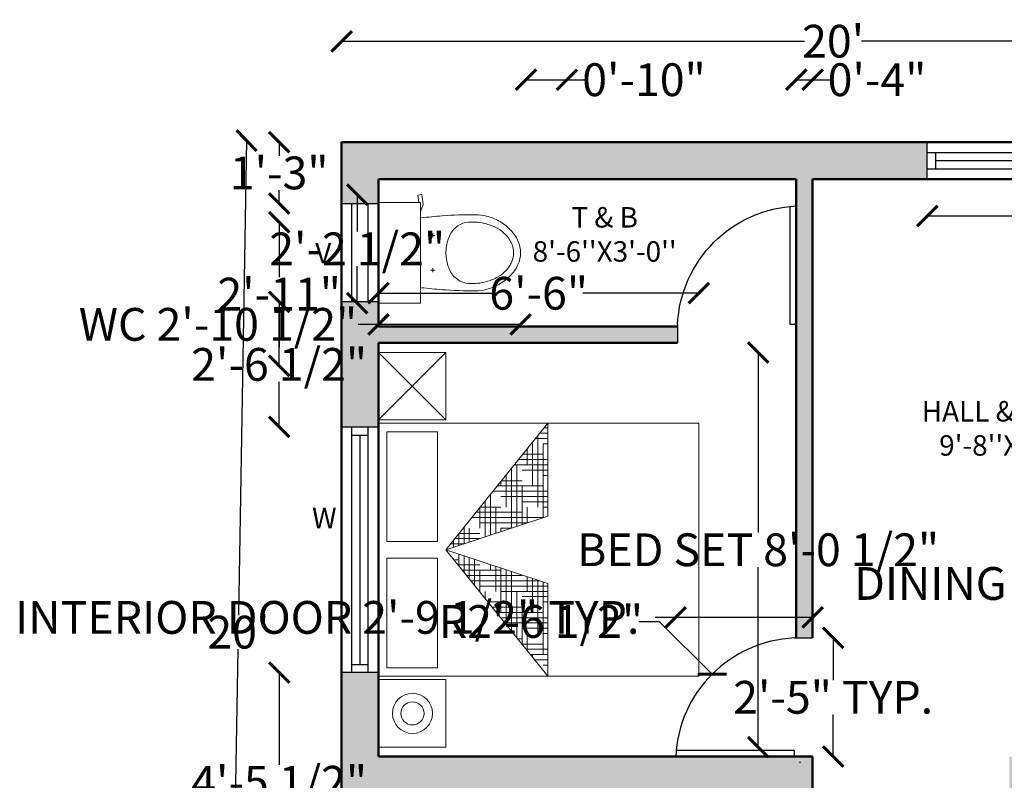
# Model space of a CAD drawing. Units: inches. Extents: x 2015 to 2400, y 1855 to 2156.
# Tile 2 of 3: x 2015 to 2255, y 1971 to 2156. Entities that reach past the tile are written whole.
import ezdxf

# ---------------------------------------------------------------- set-up
doc = ezdxf.new("R2010")
doc.units = ezdxf.units.IN
for name, color, linetype, lineweight in [('A-ANNO-DIMS', 2, 'Continuous', 18), ('A-ANNO-TEXT', 7, 'Continuous', 25), ('A-AREA-IDEN', 7, 'Continuous', 25), ('A-FLOR-FIXT', 9, 'Continuous', 18), ('A-FURN', 8, 'Continuous', 18), ('A-WALL-PATT', 30, 'Continuous', 13), ('Door', 40, 'Continuous', 25), ('Walls', 7, 'Continuous', 50), ('Windows', 150, 'Continuous', 25)]:
    doc.layers.add(name, color=color, linetype=linetype, lineweight=lineweight)
doc.styles.get("Standard").update_dxf_attribs({"font": 'arial.ttf'})
doc.dimstyles.get("Standard").update_dxf_attribs({"dimtxt": 8, "dimasz": 5, "dimexe": 0.18, "dimexo": 0.0625, "dimgap": 0.09, "dimtad": 0, "dimtih": 1, "dimtoh": 1, "dimdec": 1, "dimzin": 0, "dimdsep": 46, "dimlunit": 4, "dimtxsty": 'Standard', "dimblk": 'ARCHTICK', "dimcen": 0.09, "dimse1": 1, "dimse2": 1, "dimadec": 0, "dimazin": 0, "dimtfac": 1, "dimtdec": 1, "dimtofl": 0, "dimtmove": 0, "dimatfit": 3, "dimfxl": 1, "dimtolj": 1, "dimtzin": 0, "dimarcsym": 0})

# ---------------------------------------------------------------- blocks, each defined once
blk = doc.blocks.new('*X4')
at = {"color": 0}
for p, q in [((20.199, 14.7812), (20.2772, 14.7812)), ((20.25, 14.8125), (20.2772, 14.8125)), ((20.1487, 14.7188), (20.2772, 14.7188)), ((20.1562, 14.625), (20.1562, 14.7281)), ((20.1739, 14.75), (20.2772, 14.75)), ((20.1875, 14.75), (20.1875, 14.7669)), ((20.25, 14.3194), (20.25, 14.75)), ((20.1236, 14.6875), (20.25, 14.6875)), ((20.125, 14.5), (20.125, 14.6893)), ((20.0625, 14.2573), (20.0625, 14.6116)), ((20.0938, 14.375), (20.0938, 14.6504)), ((20.0984, 14.6562), (20.125, 14.6562)), ((20.2188, 14.3091), (20.2188, 14.625)), ((20.25, 14.625), (20.2772, 14.625)), ((20.023, 14.5625), (20.2772, 14.5625)), ((20.0312, 14.2469), (20.0312, 14.5727)), ((20.125, 14.5938), (20.2772, 14.5938)), ((19.9727, 14.5), (20.25, 14.5)), ((19.9979, 14.5312), (20.2772, 14.5312)), ((20, 14.2366), (20, 14.5)), ((20.1875, 14.2987), (20.1875, 14.5)), ((19.9225, 14.4375), (20, 14.4375)), ((19.9476, 14.4688), (20.125, 14.4688)), ((20.25, 14.4375), (20.2772, 14.4375)), ((19.875, 14.25), (19.875, 14.3785)), ((19.9062, 14.375), (19.9062, 14.4174)), ((19.9688, 14.2262), (19.9688, 14.375)), ((20, 14.375), (20.2772, 14.375)), ((20.125, 14.4062), (20.2772, 14.4062)), ((20.1562, 14.2884), (20.1562, 14.375)), ((19.8219, 14.3125), (20.2291, 14.3125)), ((19.8438, 14.1848), (19.8438, 14.3397)), ((19.875, 14.3438), (20.2772, 14.3438)), ((19.7716, 14.25), (20, 14.25)), ((19.7812, 14.1641), (19.7812, 14.262)), ((19.7967, 14.2812), (20.125, 14.2812)), ((19.8125, 14.1744), (19.8125, 14.3008)), ((19.9375, 14.2159), (19.9375, 14.25)), ((19.7465, 14.2188), (19.875, 14.2188)), ((19.75, 14.1537), (19.75, 14.2231)), ((19.7213, 14.1875), (19.75, 14.1875)), ((19.7018, 14.0938), (19.7786, 14.0938)), ((19.7188, 14.0726), (19.7188, 14.1136)), ((19.75, 14.0338), (19.75, 14.1032)), ((19.7812, 13.9949), (19.7812, 14.0929)), ((19.8125, 14), (19.8125, 14.0825)), ((19.7269, 14.0625), (19.8728, 14.0625)), ((19.752, 14.0312), (19.875, 14.0312)), ((19.9062, 13.8396), (19.9062, 14.0514)), ((19.9375, 13.8007), (19.9375, 14.0411)), ((19.9688, 13.875), (19.9688, 14.0307)), ((20, 14), (20, 14.0204)), ((19.875, 13.8784), (19.875, 14)), ((19.875, 13.9688), (20.1557, 13.9688)), ((20, 14), (20.0614, 14)), ((20.0625, 13.6454), (20.0625, 13.9996)), ((20.0938, 13.625), (20.0938, 13.9893)), ((20.125, 13.75), (20.125, 13.9789)), ((20.1562, 13.875), (20.1562, 13.9686)), ((19.8275, 13.9375), (20.25, 13.9375)), ((19.8526, 13.9062), (20.125, 13.9062)), ((20.25, 13.5), (20.25, 13.9375)), ((19.8777, 13.875), (20, 13.875)), ((20.0312, 13.6842), (20.0312, 13.875)), ((20.125, 13.8438), (20.2772, 13.8438)), ((20.2188, 13.4511), (20.2188, 13.875)), ((20.25, 13.875), (20.2772, 13.875)), ((19.9532, 13.7812), (20.2772, 13.7812)), ((20, 13.8125), (20.2772, 13.8125)), ((19.9783, 13.75), (20.25, 13.75)), ((20, 13.723), (20, 13.75)), ((20.1875, 13.49), (20.1875, 13.75)), ((20.0035, 13.7188), (20.125, 13.7188)), ((20.25, 13.6875), (20.2772, 13.6875)), ((20.0789, 13.625), (20.2772, 13.625)), ((20.125, 13.6562), (20.2772, 13.6562)), ((20.1562, 13.5288), (20.1562, 13.625)), ((20.104, 13.5938), (20.2772, 13.5938)), ((20.1292, 13.5625), (20.25, 13.5625)), ((20.25, 13.5), (20.2772, 13.5)), ((20.2046, 13.4688), (20.2772, 13.4688)), ((20.2297, 13.4375), (20.2772, 13.4375)), ((20.2549, 13.4062), (20.2772, 13.4062))]:
    blk.add_line(p, q, dxfattribs=at)
blk = doc.blocks.new('MAT-P13')
for p, q in [((-1.17, 0), (-1.17, -0.4)), ((-1.17, 0), (-0.77, 0)), ((-0.77, 0), (-0.77, -0.4)), ((-0.75, 0), (0.75, 0)), ((-0.75, 0), (-0.75, -1.9)), ((0.75, 0), (0.75, -1.9)), ((0.77, 0), (1.17, 0)), ((0.77, 0), (0.77, -0.4)), ((0.77, -0.4), (1.17, 0)), ((1.17, -0.4), (0.77, 0)), ((1.17, 0), (1.17, -0.4)), ((-0.7, -0.05), (-0.7, -0.35)), ((-0.7, -0.05), (-0.05, -0.05)), ((-0.05, -0.35), (-0.05, -0.05)), ((0.05, -0.05), (0.7, -0.05)), ((0.05, -0.35), (0.05, -0.05)), ((0.7, -0.05), (0.7, -0.35)), ((-0.7, -0.35), (-0.05, -0.35)), ((0.05, -0.35), (0.7, -0.35)), ((-1.17, -0.4), (-0.77, -0.4)), ((-0.75, -1.0034), (0, -0.4)), ((0, -0.4), (-0.75, -1.0034)), ((0, -0.4), (-0.2, -1.0034)), ((0, -0.4), (0.2, -1.0034)), ((0, -0.4), (0.75, -1.0034)), ((0.77, -0.4), (1.17, -0.4)), ((-0.75, -1.0034), (-0.2, -1.0034)), ((0.2, -1.0034), (0.75, -1.0034)), ((0.75, -1.9), (-0.75, -1.9))]:
    blk.add_line(p, q)
for radius in [0.1189, 0.0686]:
    blk.add_circle((-0.97, -0.2016), radius)
at = {"xscale": -1, "rotation": 90}
blk.add_blockref('*X4', (14.1285, 19.2738), dxfattribs=at)
blk = doc.blocks.new('AP0B05')
for p, q in [((35, 100), (35, 880)), ((75, 100), (75, 878.9)), ((35, 100), (35, -20)), ((815, 100), (815, -20))]:
    blk.add_line(p, q)
blk.add_lwpolyline([(35, 100), (75, 100)])
blk.add_arc((-2.4, 62.6), 818.3, 2.62122, 87.37878)
blk = doc.blocks.new('toilet-1')
at = {"color": 0, "linetype": 'ByBlock'}
for p, q in [((-0.23, -0.02), (-0.23, -0.2116)), ((0.23, -0.02), (-0.23, -0.02)), ((0.23, -0.02), (0.23, -0.2116)), ((-0.23, -0.2116), (0.23, -0.2116)), ((0.1917, -0.2144), (0.2206, -0.225)), ((0.2206, -0.225), (0.266, -0.2187)), ((0.2633, -0.1997), (0.23, -0.2044)), ((0.266, -0.2187), (0.2633, -0.1997)), ((-0.0889, -0.2683), (-0.0697, -0.2683)), ((-0.0793, -0.2587), (-0.0793, -0.2778)), ((0.0889, -0.2683), (0.0698, -0.2683)), ((0.0794, -0.2587), (0.0794, -0.2778)), ((0, -0.6382), (0, -0.6382))]:
    blk.add_line(p, q, dxfattribs=at)
for centre, radius, start, end in [((3.5272, -0.6239), 3.7093, 173.6925, 175.1593), ((-3.527, -0.624), 3.7093, 4.8413, 6.3171), ((1.7368, -0.4519), 1.9109, 175.7698, 180.3758), ((-1.7366, -0.4519), 1.9109, 359.6242, 4.2302), ((-0.0312, -0.4465), 0.1114, 113.8997, 145.1485), ((0, -0.5169), 0.1884, 66.0939, 113.9061), ((0.0312, -0.4465), 0.1114, 34.8515, 66.1003), ((-0.0408, -0.4398), 0.0996, 145.1497, 175.881), ((0.0409, -0.4398), 0.0996, 4.119, 34.8503), ((0.0981, -0.4497), 0.2389, 175.8862, 195.5931), ((-0.098, -0.4497), 0.2389, 344.4069, 4.1138), ((0.0353, -0.463), 0.2093, 180.3747, 194.3375), ((-0.0351, -0.463), 0.2093, 345.6614, 359.6243), ((0.055, -0.458), 0.2297, 194.3353, 209.622), ((0.0961, -0.4503), 0.2369, 195.5969, 209.3771), ((-0.096, -0.4503), 0.2369, 330.6229, 344.4031), ((-0.0548, -0.458), 0.2297, 330.3788, 345.6655), ((0.0647, -0.4524), 0.2409, 209.6273, 224.5489), ((0.0232, -0.4913), 0.1532, 209.3871, 226.5438), ((-0.0231, -0.4913), 0.1532, 313.4562, 330.6129), ((-0.0645, -0.4524), 0.2409, 315.4504, 330.372), ((0.0178, -0.4986), 0.1751, 224.552, 245.714), ((0.0152, -0.4997), 0.1416, 226.5501, 246.5527), ((0, -0.5347), 0.1034, 246.5493, 270.0042), ((0, -0.5347), 0.1034, 269.9958, 293.4507), ((-0.0151, -0.4997), 0.1416, 293.4473, 313.4499), ((-0.0176, -0.4986), 0.1751, 294.2865, 315.4485), ((0.0004, -0.538), 0.132, 245.5845, 269.8782), ((-0.0002, -0.538), 0.132, 270.1216, 294.4153)]:
    blk.add_arc(centre, radius, start, end, dxfattribs=at)
blk = doc.blocks.new('_ArchTick')
at = {"color": 0, "linetype": 'ByBlock', "const_width": 0.15}
blk.add_lwpolyline([(-0.5, -0.5), (0.5, 0.5)], dxfattribs=at)
blk = doc.blocks.new('*D12')
at = {"layer": 'A-ANNO-DIMS', "color": 0, "lineweight": -2, "transparency": 16777216}
for p, q in [((2093.14, 2151.23), (2206.19, 2151.23)), ((2333.14, 2151.23), (2220.09, 2151.23))]:
    blk.add_line(p, q, dxfattribs=at)
at = {"layer": 'Defpoints', "color": 0, "transparency": 16777216}
for p in [(2333.14, 2151.23), (2093.14, 2126.58), (2333.14, 2126.58)]:
    blk.add_point(p, dxfattribs=at)
at = {"layer": 'A-ANNO-DIMS', "color": 0, "lineweight": -2, "transparency": 16777216, "xscale": 5, "yscale": 5, "zscale": 5, "rotation": 180}
blk.add_blockref('_ArchTick', (2093.14, 2151.23), dxfattribs=at)
at = {"layer": 'A-ANNO-DIMS', "color": 0, "lineweight": -2, "transparency": 16777216, "xscale": 5, "yscale": 5, "zscale": 5}
blk.add_blockref('_ArchTick', (2333.14, 2151.23), dxfattribs=at)
at = {"layer": 'A-ANNO-DIMS', "color": 0, "transparency": 16777216, "insert": (2213.14, 2151.23), "char_height": 8, "attachment_point": 5}
blk.add_mtext("\\A1;20'", dxfattribs=at)
blk = doc.blocks.new('*D13')
at = {"layer": 'A-ANNO-DIMS', "color": 0, "lineweight": -2, "transparency": 16777216}
for p, q in [((2069.93, 2126.97), (2067.99, 2011.14)), ((2065.91, 1886.97), (2067.85, 2002.79))]:
    blk.add_line(p, q, dxfattribs=at)
at = {"layer": 'Defpoints', "color": 0, "transparency": 16777216}
for p in [(2093.14, 2126.58), (2065.91, 1886.97), (2089.12, 1886.58)]:
    blk.add_point(p, dxfattribs=at)
at = {"layer": 'A-ANNO-DIMS', "color": 0, "lineweight": -2, "transparency": 16777216, "xscale": 5, "yscale": 5, "zscale": 5}
for p, rotation in [((2069.93, 2126.97), 89.03988190259393), ((2065.91, 1886.97), 269.039881902594)]:
    blk.add_blockref('_ArchTick', p, dxfattribs=dict(at, rotation=rotation))
at = {"layer": 'A-ANNO-DIMS', "color": 0, "transparency": 16777216, "insert": (2067.92, 2006.97), "char_height": 8, "attachment_point": 5}
blk.add_mtext("\\A1;20'", dxfattribs=at)
blk = doc.blocks.new('WIN-60IN')
for p, q in [((0, 6.5), (60, 6.5)), ((2, 6.5), (2, 2.5)), ((58, 6.5), (58, 2.5)), ((0, 2.5), (60, 2.5)), ((2, 4.5), (58, 4.5))]:
    blk.add_line(p, q)
blk.add_lwpolyline([(0, 9), (60, 9), (60, 0), (0, 0)], close=True)
blk = doc.blocks.new('WIN-24IN')
for p, q in [((2.5, 0), (2.5, 24)), ((6.5, 0), (6.5, 24))]:
    blk.add_line(p, q)
blk.add_lwpolyline([(0, 0), (0, 24), (9, 24), (9, 0)], close=True)
blk = doc.blocks.new('*D17')
at = {"layer": 'A-ANNO-DIMS', "color": 0, "lineweight": -2, "transparency": 16777216}
for p, q in [((2174.71, 2010.57), (2169.71, 2010.57)), ((2208.14, 2010.57), (2174.71, 2010.57))]:
    blk.add_line(p, q, dxfattribs=at)
at = {"layer": 'Defpoints', "color": 0, "transparency": 16777216}
for p in [(2174.71, 2010.57), (2174.71, 2005.56), (2208.14, 2005.56)]:
    blk.add_point(p, dxfattribs=at)
at = {"layer": 'A-ANNO-DIMS', "color": 0, "lineweight": -2, "transparency": 16777216, "xscale": 5, "yscale": 5, "zscale": 5, "rotation": 180}
blk.add_blockref('_ArchTick', (2174.71, 2010.57), dxfattribs=at)
at = {"layer": 'A-ANNO-DIMS', "color": 0, "lineweight": -2, "transparency": 16777216, "xscale": 5, "yscale": 5, "zscale": 5}
blk.add_blockref('_ArchTick', (2208.14, 2010.57), dxfattribs=at)
at = {"layer": 'A-ANNO-DIMS', "color": 0, "transparency": 16777216, "insert": (2089.64, 2010.57), "char_height": 8, "attachment_point": 5}
blk.add_mtext('\\A1;INTERIOR DOOR 2\'-9 1/2" TYP.', dxfattribs=at)
blk = doc.blocks.new('*D18')
at = {"layer": 'A-ANNO-DIMS', "color": 0, "lineweight": -2, "transparency": 16777216}
for p, q in [((2213.15, 2005.56), (2213.15, 1995.24)), ((2213.15, 1976.58), (2213.15, 1986.89))]:
    blk.add_line(p, q, dxfattribs=at)
at = {"layer": 'Defpoints', "color": 0, "transparency": 16777216}
for p in [(2208.14, 2005.56), (2213.15, 2005.56), (2208.14, 1976.58)]:
    blk.add_point(p, dxfattribs=at)
at = {"layer": 'A-ANNO-DIMS', "color": 0, "lineweight": -2, "transparency": 16777216, "xscale": 5, "yscale": 5, "zscale": 5}
for p, rotation in [((2213.15, 2005.56), 90), ((2213.15, 1976.58), 270)]:
    blk.add_blockref('_ArchTick', p, dxfattribs=dict(at, rotation=rotation))
at = {"layer": 'A-ANNO-DIMS', "color": 0, "transparency": 16777216, "insert": (2213.15, 1991.07), "char_height": 8, "attachment_point": 5}
blk.add_mtext('\\A1;2\'-5" TYP.', dxfattribs=at)
blk = doc.blocks.new('*D19')
at = {"layer": 'A-ANNO-DIMS', "color": 0, "lineweight": -2, "transparency": 16777216}
for p, q in [((2236.14, 2108.58), (2296.14, 2108.58)), ((2296.14, 2108.58), (2301.14, 2108.58))]:
    blk.add_line(p, q, dxfattribs=at)
at = {"layer": 'Defpoints', "color": 0, "transparency": 16777216}
for p in [(2236.14, 2117.58), (2296.14, 2117.58), (2296.14, 2108.58)]:
    blk.add_point(p, dxfattribs=at)
at = {"layer": 'A-ANNO-DIMS', "color": 0, "lineweight": -2, "transparency": 16777216, "xscale": 5, "yscale": 5, "zscale": 5, "rotation": 180}
blk.add_blockref('_ArchTick', (2236.14, 2108.58), dxfattribs=at)
at = {"layer": 'A-ANNO-DIMS', "color": 0, "lineweight": -2, "transparency": 16777216, "xscale": 5, "yscale": 5, "zscale": 5}
blk.add_blockref('_ArchTick', (2296.14, 2108.58), dxfattribs=at)
at = {"layer": 'A-ANNO-DIMS', "color": 0, "transparency": 16777216, "insert": (2351.85, 2108.58), "char_height": 8, "attachment_point": 5}
blk.add_mtext('\\A1;WINDOW 5\'-0" TYP.', dxfattribs=at)
blk = doc.blocks.new('*D27')
at = {"layer": 'A-ANNO-DIMS', "color": 0, "lineweight": -2, "transparency": 16777216}
for p, q in [((2264.14, 2047.98), (2264.14, 2023.08)), ((2264.14, 1989.73), (2264.14, 2014.63))]:
    blk.add_line(p, q, dxfattribs=at)
at = {"layer": 'Defpoints', "color": 0, "transparency": 16777216}
for p in [(2264.14, 2047.98), (2272.88, 2047.98), (2272.88, 1989.73)]:
    blk.add_point(p, dxfattribs=at)
at = {"layer": 'A-ANNO-DIMS', "color": 0, "lineweight": -2, "transparency": 16777216, "xscale": 5, "yscale": 5, "zscale": 5}
for p, rotation in [((2264.14, 2047.98), 90), ((2264.14, 1989.73), 270)]:
    blk.add_blockref('_ArchTick', p, dxfattribs=dict(at, rotation=rotation))
at = {"layer": 'A-ANNO-DIMS', "color": 0, "transparency": 16777216, "insert": (2264.14, 2018.85), "char_height": 8, "attachment_point": 5}
blk.add_mtext('\\A1;DINING SET 4\'-10"', dxfattribs=at)
blk = doc.blocks.new('*D31')
at = {"layer": 'A-ANNO-DIMS', "color": 0, "lineweight": -2, "transparency": 16777216}
for p, q in [((2194.82, 2075.25), (2194.82, 2031.31)), ((2194.82, 1978.91), (2194.82, 2022.85))]:
    blk.add_line(p, q, dxfattribs=at)
at = {"layer": 'Defpoints', "color": 0, "transparency": 16777216}
for p in [(2180.36, 2075.25), (2194.82, 2075.25), (2180.36, 1978.91)]:
    blk.add_point(p, dxfattribs=at)
at = {"layer": 'A-ANNO-DIMS', "color": 0, "lineweight": -2, "transparency": 16777216, "xscale": 5, "yscale": 5, "zscale": 5}
for p, rotation in [((2194.82, 2075.25), 90), ((2194.82, 1978.91), 270)]:
    blk.add_blockref('_ArchTick', p, dxfattribs=dict(at, rotation=rotation))
at = {"layer": 'A-ANNO-DIMS', "color": 0, "transparency": 16777216, "insert": (2194.82, 2027.08), "char_height": 8, "attachment_point": 5}
blk.add_mtext('\\A1;BED SET 8\'-0 1/2"', dxfattribs=at)
blk = doc.blocks.new('*D32')
at = {"layer": 'A-ANNO-DIMS', "color": 0, "lineweight": -2, "transparency": 16777216}
for p, q in [((2102.14, 2089.7), (2130.51, 2089.7)), ((2180.36, 2089.7), (2152, 2089.7))]:
    blk.add_line(p, q, dxfattribs=at)
at = {"layer": 'Defpoints', "color": 0, "transparency": 16777216}
for p in [(2102.14, 2089.7), (2102.14, 2075.25), (2180.36, 2075.25)]:
    blk.add_point(p, dxfattribs=at)
at = {"layer": 'A-ANNO-DIMS', "color": 0, "lineweight": -2, "transparency": 16777216, "xscale": 5, "yscale": 5, "zscale": 5, "rotation": 180}
blk.add_blockref('_ArchTick', (2102.14, 2089.7), dxfattribs=at)
at = {"layer": 'A-ANNO-DIMS', "color": 0, "lineweight": -2, "transparency": 16777216, "xscale": 5, "yscale": 5, "zscale": 5}
blk.add_blockref('_ArchTick', (2180.36, 2089.7), dxfattribs=at)
at = {"layer": 'A-ANNO-DIMS', "color": 0, "transparency": 16777216, "insert": (2141.25, 2089.7), "char_height": 8, "attachment_point": 5}
blk.add_mtext('\\A1;6\'-6"', dxfattribs=at)
blk = doc.blocks.new('*D33')
at = {"layer": 'A-ANNO-DIMS', "color": 0, "lineweight": -2, "transparency": 16777216}
for p, q in [((2102.14, 2082.11), (2097.14, 2082.11)), ((2136.82, 2082.11), (2102.14, 2082.11))]:
    blk.add_line(p, q, dxfattribs=at)
at = {"layer": 'Defpoints', "color": 0, "transparency": 16777216}
for p in [(2102.14, 2087.31), (2136.82, 2087.31), (2102.14, 2082.11)]:
    blk.add_point(p, dxfattribs=at)
at = {"layer": 'A-ANNO-DIMS', "color": 0, "lineweight": -2, "transparency": 16777216, "xscale": 5, "yscale": 5, "zscale": 5, "rotation": 180}
blk.add_blockref('_ArchTick', (2102.14, 2082.11), dxfattribs=at)
at = {"layer": 'A-ANNO-DIMS', "color": 0, "lineweight": -2, "transparency": 16777216, "xscale": 5, "yscale": 5, "zscale": 5}
blk.add_blockref('_ArchTick', (2136.82, 2082.11), dxfattribs=at)
at = {"layer": 'A-ANNO-DIMS', "color": 0, "transparency": 16777216, "insert": (2062.96, 2082.11), "char_height": 8, "attachment_point": 5}
blk.add_mtext('\\A1;WC 2\'-10 1/2"', dxfattribs=at)
blk = doc.blocks.new('*D34')
at = {"layer": 'A-ANNO-DIMS', "color": 0, "lineweight": -2, "transparency": 16777216}
for p, q in [((2096.94, 2113.77), (2096.94, 2104.77)), ((2096.94, 2087.31), (2096.94, 2096.31))]:
    blk.add_line(p, q, dxfattribs=at)
at = {"layer": 'Defpoints', "color": 0, "transparency": 16777216}
for p in [(2096.94, 2113.77), (2102.14, 2113.77), (2102.14, 2087.31)]:
    blk.add_point(p, dxfattribs=at)
at = {"layer": 'A-ANNO-DIMS', "color": 0, "lineweight": -2, "transparency": 16777216, "xscale": 5, "yscale": 5, "zscale": 5}
for p, rotation in [((2096.94, 2113.77), 90), ((2096.94, 2087.31), 270)]:
    blk.add_blockref('_ArchTick', p, dxfattribs=dict(at, rotation=rotation))
at = {"layer": 'A-ANNO-DIMS', "color": 0, "transparency": 16777216, "insert": (2096.94, 2100.54), "char_height": 8, "attachment_point": 5}
blk.add_mtext('\\A1;2\'-2 1/2"', dxfattribs=at)
blk = doc.blocks.new('*D40')
at = {"layer": 'A-ANNO-DIMS', "color": 0, "lineweight": -2, "transparency": 16777216}
for p, q in [((2077.89, 2087.58), (2077.89, 2076.56)), ((2077.89, 2057.08), (2077.89, 2068.1))]:
    blk.add_line(p, q, dxfattribs=at)
at = {"layer": 'Defpoints', "color": 0, "transparency": 16777216}
for p in [(2077.89, 2087.58), (2093.14, 2087.58), (2093.14, 2057.08)]:
    blk.add_point(p, dxfattribs=at)
at = {"layer": 'A-ANNO-DIMS', "color": 0, "lineweight": -2, "transparency": 16777216, "xscale": 5, "yscale": 5, "zscale": 5}
for p, rotation in [((2077.89, 2087.58), 90), ((2077.89, 2057.08), 270)]:
    blk.add_blockref('_ArchTick', p, dxfattribs=dict(at, rotation=rotation))
at = {"layer": 'A-ANNO-DIMS', "color": 0, "transparency": 16777216, "insert": (2077.89, 2072.33), "char_height": 8, "attachment_point": 5}
blk.add_mtext('\\A1;2\'-6 1/2"', dxfattribs=at)
blk = doc.blocks.new('*D41')
at = {"layer": 'A-ANNO-DIMS', "color": 0, "lineweight": -2, "transparency": 16777216}
for p, q in [((2077.89, 1997.08), (2077.89, 1974.56)), ((2077.89, 1943.58), (2077.89, 1966.1))]:
    blk.add_line(p, q, dxfattribs=at)
at = {"layer": 'Defpoints', "color": 0, "transparency": 16777216}
for p in [(2077.89, 1997.08), (2093.14, 1997.08), (2093.14, 1943.58)]:
    blk.add_point(p, dxfattribs=at)
at = {"layer": 'A-ANNO-DIMS', "color": 0, "lineweight": -2, "transparency": 16777216, "xscale": 5, "yscale": 5, "zscale": 5}
for p, rotation in [((2077.89, 1997.08), 90), ((2077.89, 1943.58), 270)]:
    blk.add_blockref('_ArchTick', p, dxfattribs=dict(at, rotation=rotation))
at = {"layer": 'A-ANNO-DIMS', "color": 0, "transparency": 16777216, "insert": (2077.89, 1970.33), "char_height": 8, "attachment_point": 5}
blk.add_mtext('\\A1;4\'-5 1/2"', dxfattribs=at)
blk = doc.blocks.new('*D42')
at = {"layer": 'A-ANNO-DIMS', "color": 0, "lineweight": -2, "transparency": 16777216}
for p, q in [((2077.89, 2126.58), (2077.89, 2123.26)), ((2077.89, 2111.58), (2077.89, 2114.9))]:
    blk.add_line(p, q, dxfattribs=at)
at = {"layer": 'Defpoints', "color": 0, "transparency": 16777216}
for p in [(2077.89, 2126.58), (2093.14, 2126.58), (2093.14, 2111.58)]:
    blk.add_point(p, dxfattribs=at)
at = {"layer": 'A-ANNO-DIMS', "color": 0, "lineweight": -2, "transparency": 16777216, "xscale": 5, "yscale": 5, "zscale": 5}
for p, rotation in [((2077.89, 2126.58), 90), ((2077.89, 2111.58), 270)]:
    blk.add_blockref('_ArchTick', p, dxfattribs=dict(at, rotation=rotation))
at = {"layer": 'A-ANNO-DIMS', "color": 0, "transparency": 16777216, "insert": (2077.89, 2119.08), "char_height": 8, "attachment_point": 5}
blk.add_mtext('\\A1;1\'-3"', dxfattribs=at)
blk = doc.blocks.new('*D43')
at = {"layer": 'A-ANNO-DIMS', "color": 0, "lineweight": -2, "transparency": 16777216}
for p, q in [((2138.14, 2141.83), (2148.14, 2141.83)), ((2148.14, 2141.83), (2153.14, 2141.83))]:
    blk.add_line(p, q, dxfattribs=at)
at = {"layer": 'Defpoints', "color": 0, "transparency": 16777216}
for p in [(2148.14, 2141.83), (2138.14, 1895.58), (2148.14, 1895.58)]:
    blk.add_point(p, dxfattribs=at)
at = {"layer": 'A-ANNO-DIMS', "color": 0, "lineweight": -2, "transparency": 16777216, "xscale": 5, "yscale": 5, "zscale": 5, "rotation": 180}
blk.add_blockref('_ArchTick', (2138.14, 2141.83), dxfattribs=at)
at = {"layer": 'A-ANNO-DIMS', "color": 0, "lineweight": -2, "transparency": 16777216, "xscale": 5, "yscale": 5, "zscale": 5}
blk.add_blockref('_ArchTick', (2148.14, 2141.83), dxfattribs=at)
at = {"layer": 'A-ANNO-DIMS', "color": 0, "transparency": 16777216, "insert": (2166.97, 2141.83), "char_height": 8, "attachment_point": 5}
blk.add_mtext('\\A1;0\'-10"', dxfattribs=at)
blk = doc.blocks.new('*D50')
at = {"layer": 'A-ANNO-DIMS', "color": 0, "lineweight": -2, "transparency": 16777216}
for p, q in [((2077.89, 2107.02), (2077.89, 2093.6)), ((2077.89, 2071.97), (2077.89, 2085.39))]:
    blk.add_line(p, q, dxfattribs=at)
at = {"layer": 'Defpoints', "color": 0, "transparency": 16777216}
for p in [(2077.89, 2107.02), (2279.88, 2107.02), (2279.88, 2071.97)]:
    blk.add_point(p, dxfattribs=at)
at = {"layer": 'A-ANNO-DIMS', "color": 0, "lineweight": -2, "transparency": 16777216, "xscale": 5, "yscale": 5, "zscale": 5}
for p, rotation in [((2077.89, 2107.02), 90), ((2077.89, 2071.97), 270)]:
    blk.add_blockref('_ArchTick', p, dxfattribs=dict(at, rotation=rotation))
at = {"layer": 'A-ANNO-DIMS', "color": 0, "transparency": 16777216, "insert": (2077.89, 2089.49), "char_height": 8, "attachment_point": 5}
blk.add_mtext('\\A1;2\'-11"', dxfattribs=at)
blk = doc.blocks.new('*D53')
at = {"layer": 'A-ANNO-DIMS', "color": 0, "lineweight": -2, "transparency": 16777216}
for p, q in [((2204.14, 2141.83), (2208.14, 2141.83)), ((2208.14, 2141.83), (2213.14, 2141.83))]:
    blk.add_line(p, q, dxfattribs=at)
at = {"layer": 'Defpoints', "color": 0, "transparency": 16777216}
for p in [(2208.14, 2141.83), (2204.14, 2117.58), (2208.14, 2117.58)]:
    blk.add_point(p, dxfattribs=at)
at = {"layer": 'A-ANNO-DIMS', "color": 0, "lineweight": -2, "transparency": 16777216, "xscale": 5, "yscale": 5, "zscale": 5, "rotation": 180}
blk.add_blockref('_ArchTick', (2204.14, 2141.83), dxfattribs=at)
at = {"layer": 'A-ANNO-DIMS', "color": 0, "lineweight": -2, "transparency": 16777216, "xscale": 5, "yscale": 5, "zscale": 5}
blk.add_blockref('_ArchTick', (2208.14, 2141.83), dxfattribs=at)
at = {"layer": 'A-ANNO-DIMS', "color": 0, "transparency": 16777216, "insert": (2223.86, 2141.83), "char_height": 8, "attachment_point": 5}
blk.add_mtext('\\A1;0\'-4"', dxfattribs=at)
blk = doc.blocks.new('*D54')
at = {"layer": 'A-ANNO-DIMS', "color": 0, "lineweight": -2, "transparency": 16777216}
for p, q in [((2165.68, 2009.58), (2170.68, 2009.58)), ((2170.68, 2009.58), (2183.58, 1996.68)), ((2204.98, 1975.19), (2205.16, 1975.19)), ((2205.07, 1975.1), (2205.07, 1975.28))]:
    blk.add_line(p, q, dxfattribs=at)
at = {"layer": 'Defpoints', "color": 0, "transparency": 16777216}
for p in [(2183.58, 1996.68), (2205.07, 1975.19)]:
    blk.add_point(p, dxfattribs=at)
at = {"layer": 'A-ANNO-DIMS', "color": 0, "lineweight": -2, "transparency": 16777216, "xscale": 5, "yscale": 5, "zscale": 5, "rotation": 315.0005984440339}
blk.add_blockref('_ArchTick', (2183.58, 1996.68), dxfattribs=at)
at = {"layer": 'A-ANNO-DIMS', "color": 0, "transparency": 16777216, "insert": (2141.81, 2009.58), "char_height": 8, "attachment_point": 5}
blk.add_mtext('\\A1;R2\'-6 1/2"', dxfattribs=at)

msp = doc.modelspace()

# ---------------------------------------------------------------- hatches: boundary and pattern name
at = {"layer": 'A-WALL-PATT'}
h = msp.add_hatch(color=256, dxfattribs=at)
h.dxf.hatch_style = 1
h.paths.add_polyline_path([(2236.14, 2126.58), (2093.14, 2126.58), (2093.14, 2111.58), (2102.14, 2111.58), (2102.14, 2111.85), (2102.14, 2117.58), (2204.14, 2117.58), (2204.14, 2005.56), (2208.14, 2005.56), (2208.14, 2117.58), (2236.14, 2117.58)])
h.paths.add_polyline_path([(2102.14, 2077.58), (2175.16, 2077.58), (2175.16, 2081.58), (2102.14, 2081.58), (2102.14, 2087.58), (2093.14, 2087.58), (2093.14, 2057.08), (2102.14, 2057.08), (2102.14, 2057.96)], flags=17)
h.paths.add_polyline_path([(2208.14, 1976.58), (2203.68, 1976.58), (2174.71, 1976.58), (2102.14, 1976.58), (2102.14, 1997.08), (2093.14, 1997.08), (2093.14, 1943.58), (2102.14, 1943.58), (2102.14, 1967.58), (2208.14, 1967.58)])
h.paths.add_polyline_path([(2260.14, 1976.58), (2256.14, 1976.58), (2256.14, 1886.58), (2262.02, 1886.58), (2262.02, 1895.58), (2260.14, 1895.58)])
h.paths.add_polyline_path([(2208.14, 1895.58), (2102.14, 1895.58), (2102.14, 1919.58), (2093.14, 1919.58), (2093.14, 1886.58), (2208.14, 1886.58)])

# ---------------------------------------------------------------- linework, layer by layer
at = {"layer": 'Walls'}
for p, q in [((2093.14, 2126.58), (2333.14, 2126.58)), ((2093.14, 2126.58), (2093.14, 1886.58)), ((2102.14, 2117.58), (2204.14, 2117.58)), ((2102.14, 2117.58), (2102.14, 2081.58)), ((2204.14, 2117.58), (2204.14, 2005.56)), ((2208.14, 2117.58), (2208.14, 2005.56)), ((2208.14, 2117.58), (2324.14, 2117.58)), ((2102.14, 2081.58), (2175.16, 2081.58)), ((2102.14, 2077.58), (2175.16, 2077.58)), ((2102.14, 2077.58), (2102.14, 1976.58)), ((2102.14, 1976.58), (2208.14, 1976.58)), ((2208.14, 1976.58), (2208.14, 1967.58))]:
    msp.add_line(p, q, dxfattribs=at)

# ---------------------------------------------------------------- block references
at = {"layer": 'A-FLOR-FIXT', "xscale": 53.35698818414478, "yscale": 53.35698818414478, "zscale": 53.35698818414478, "rotation": 90}
msp.add_blockref('toilet-1', (2101.07, 2099.58), dxfattribs=at)
at = {"layer": 'A-FURN', "xscale": 41.17100610299669, "yscale": 41.17100610299669, "zscale": 41.17100610299669, "rotation": 90}
msp.add_blockref('MAT-P13', (2102.14, 2027.08), dxfattribs=at)
at = {"layer": 'Door', "xscale": -0.0371474756206669, "yscale": 0.0371474756206669, "zscale": 0.0371474756206669}
msp.add_blockref('AP0B05', (2205.44, 2078.32), dxfattribs=at)
at = {"layer": 'Door', "xscale": 0.0371474756206669, "yscale": 0.0371474756206669, "zscale": 0.0371474756206669, "rotation": 90}
msp.add_blockref('AP0B05', (2207.4, 1975.28), dxfattribs=at)
at = {"layer": 'Windows'}
for name, p in [('WIN-60IN', (2236.14, 2117.58)), ('WIN-24IN', (2093.14, 2087.58))]:
    msp.add_blockref(name, p, dxfattribs=at)
at = {"layer": 'Windows', "rotation": 90.00000000000216}
msp.add_blockref('WIN-60IN', (2102.14, 1997.08), dxfattribs=at)

# ---------------------------------------------------------------- texts
at = {"layer": 'A-ANNO-TEXT', "char_height": 5, "attachment_point": 1}
for s, insert in [('\\pxqc;V', (2073.13, 2102)), ('\\pxqc;W', (2073.39, 2037.32))]:
    msp.add_mtext_dynamic_manual_height_columns(s, width=31.0576, gutter_width=12.5, heights=[0], dxfattribs=dict(at, insert=insert))
at = {"layer": 'A-AREA-IDEN', "char_height": 5, "attachment_point": 1}
for s, width, heights, insert in [("\\pxqc;T & B\\P8'-6''X3'-0''", 31.0576, [0], (2141.83, 2110.74)), ("\\pxqc;HALL & DINING\\P9'-8''X11'-9''", 54.9856, [15.52], (2231.02, 2063.39))]:
    msp.add_mtext_dynamic_manual_height_columns(s, width=width, gutter_width=12.5, heights=heights, dxfattribs=dict(at, insert=insert))

# ---------------------------------------------------------------- dimensions: what is measured, and where the dimension line sits
at = {"layer": 'A-ANNO-DIMS'}
for base, p1, p2, override, picture, middle in [((2333.14, 2151.23), (2093.14, 2126.58), (2333.14, 2126.58), {"dimclrd": 0, "dimclre": 0, "dimclrt": 0}, '*D12', (2213.14, 2151.23)), ((2148.14, 2141.83), (2138.14, 1895.58), (2148.14, 1895.58), {"dimdec": 1, "dimlfac": 1, "dimrnd": 0, "dimzin": 1, "dimdsep": 46, "dimlunit": 4, "dimfrac": 2}, '*D43', (2166.97, 2141.83)), ((2208.14, 2141.83), (2204.14, 2117.58), (2208.14, 2117.58), {"dimdec": 1, "dimlfac": 1, "dimrnd": 0, "dimzin": 1, "dimdsep": 46, "dimlunit": 4, "dimfrac": 2}, '*D53', (2223.86, 2141.83))]:
    dim = msp.add_linear_dim(base=base, p1=p1, p2=p2, dimstyle='Standard', override=override, dxfattribs=at)
    dim.commit()
    dim.dimension.update_dxf_attribs({"geometry": picture, "text_midpoint": middle})
dim = msp.add_aligned_dim(p1=(2093.14, 2126.58), p2=(2089.12, 1886.58), distance=-23.21, dimstyle='Standard', override={"dimclrd": 0, "dimclre": 0, "dimclrt": 0}, dxfattribs=at)
dim.commit()
dim.dimension.update_dxf_attribs({"geometry": '*D13', "text_midpoint": (2067.92, 2006.97)})
for base, p1, p2, angle, picture, middle in [((2077.89, 2126.58), (2093.14, 2111.58), (2093.14, 2126.58), 90, '*D42', (2077.89, 2119.08)), ((2096.94, 2113.77), (2102.14, 2087.31), (2102.14, 2113.77), 90, '*D34', (2096.94, 2100.54)), ((2077.8897, 2107.0163), (2279.8803, 2071.9679), (2279.8803, 2107.0163), 90, '*D50', (2077.8897, 2089.4921)), ((2102.14, 2089.7), (2180.36, 2075.25), (2102.14, 2075.25), 180, '*D32', (2141.25, 2089.7)), ((2077.89, 2087.58), (2093.14, 2057.08), (2093.14, 2087.58), 90, '*D40', (2077.89, 2072.33)), ((2077.89, 1997.08), (2093.14, 1943.58), (2093.14, 1997.08), 90, '*D41', (2077.89, 1970.33))]:
    dim = msp.add_linear_dim(base=base, p1=p1, p2=p2, angle=angle, dimstyle='Standard', override={"dimdec": 1, "dimlfac": 1, "dimrnd": 0, "dimzin": 1, "dimdsep": 46, "dimlunit": 4, "dimfrac": 2}, dxfattribs=at)
    dim.commit()
    dim.dimension.update_dxf_attribs({"geometry": picture, "text_midpoint": middle})
dim = msp.add_linear_dim(base=(2296.14, 2108.58), p1=(2236.14, 2117.58), p2=(2296.14, 2117.58), text='WINDOW <> TYP.', dimstyle='Standard', override={"dimdec": 1, "dimlfac": 1, "dimrnd": 0, "dimzin": 1, "dimdsep": 46, "dimlunit": 4, "dimfrac": 2}, dxfattribs=at)
dim.commit()
dim.dimension.update_dxf_attribs({"geometry": '*D19', "text_midpoint": (2351.85, 2108.58)})
for base, p1, p2, angle, text, picture, middle in [((2102.14, 2082.11), (2136.82, 2087.31), (2102.14, 2087.31), 180, 'WC <>', '*D33', (2062.96, 2082.11)), ((2194.82, 2075.25), (2180.36, 1978.91), (2180.36, 2075.25), 90, 'BED SET <>', '*D31', (2194.82, 2027.08)), ((2264.1381, 2047.976), (2272.8755, 1989.7271), (2272.8755, 2047.976), 90, 'DINING SET <>', '*D27', (2264.1381, 2018.8516)), ((2174.71, 2010.57), (2208.14, 2005.56), (2174.71, 2005.56), 180, 'INTERIOR DOOR <> TYP.', '*D17', (2089.64, 2010.57)), ((2213.15, 2005.56), (2208.14, 1976.58), (2208.14, 2005.56), 90, '<> TYP.', '*D18', (2213.15, 1991.07))]:
    dim = msp.add_linear_dim(base=base, p1=p1, p2=p2, angle=angle, text=text, dimstyle='Standard', override={"dimdec": 1, "dimlfac": 1, "dimrnd": 0, "dimzin": 1, "dimdsep": 46, "dimlunit": 4, "dimfrac": 2}, dxfattribs=at)
    dim.commit()
    dim.dimension.update_dxf_attribs({"geometry": picture, "text_midpoint": middle})
dim = msp.add_radius_dim(center=(2205.07, 1975.19), mpoint=(2183.58, 1996.68), dimstyle='Standard', override={"dimdec": 1, "dimlfac": 1, "dimrnd": 0, "dimzin": 1, "dimdsep": 46, "dimlunit": 4, "dimfrac": 2}, dxfattribs=at)
dim.commit()
dim.dimension.update_dxf_attribs({"geometry": '*D54', "text_midpoint": (2141.81, 2009.58), "dimtype": 164})

doc.saveas('drawing.dxf')
